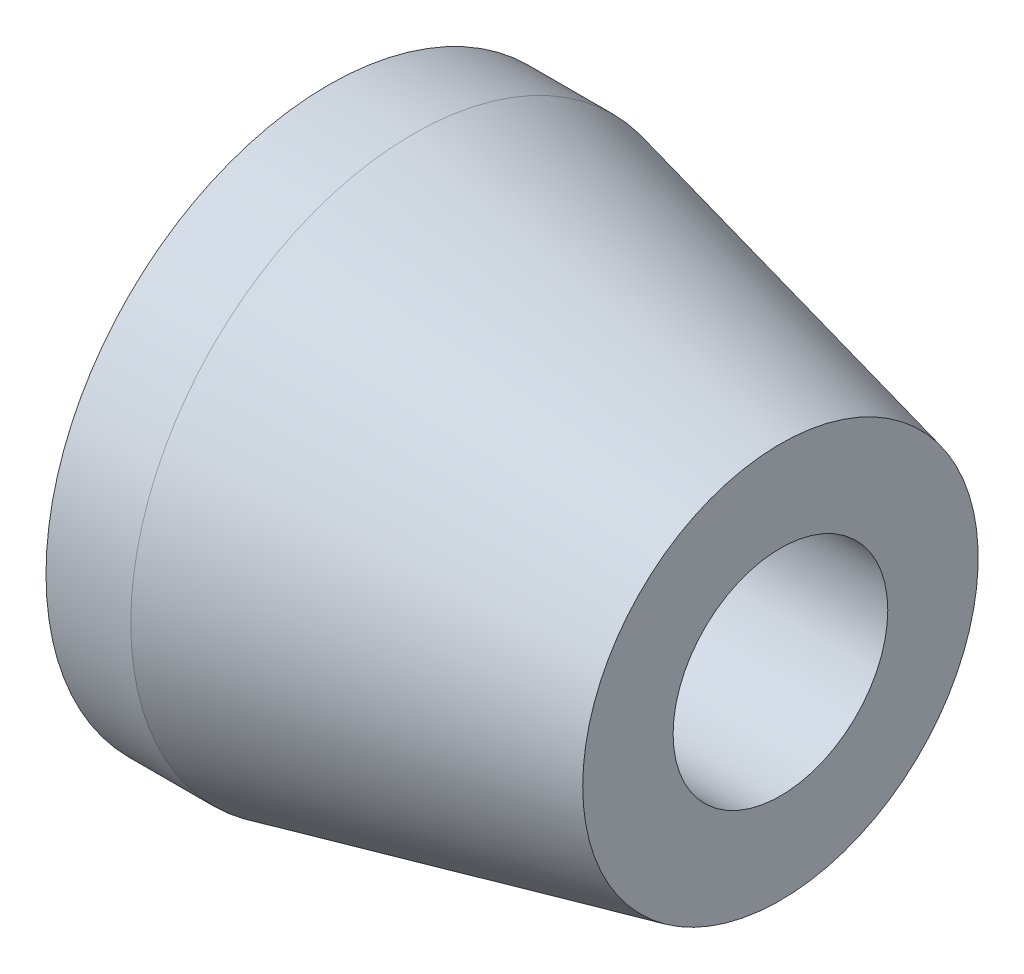
from build123d import *

# Parameters (mm, degrees)
BORE_SKETCH_R      = 3.8
THROUGH_BORE_DEPTH = 22.354156504
RECESS_SKETCH_13_R = 6.5
RECESS_13X2_DEPTH  = 2


with BuildPart() as part:
    # Bush Profile Sketch → Bush Body (revolve)
    with BuildSketch(Plane.XY, mode=Mode.PRIVATE) as bush_body_sk:
        Polygon((0, 0), (0, 10), (3, 10), (16, 7), (16, 0), align=None)
    revolve(bush_body_sk.sketch.rotate(Axis((-1000, 0, 0), (1, 0, 0)), 90), axis=Axis((-1000, 0, 0), (1, 0, 0)))

    # Bore Sketch → Through Bore (cut, through all)
    with BuildSketch(Plane.ZY):
        Circle(BORE_SKETCH_R)
    extrude(amount=-THROUGH_BORE_DEPTH, mode=Mode.SUBTRACT)

    # Recess Sketch Ø13 → Recess Ø13x2 (cut)
    with BuildSketch(Plane.ZY):
        Circle(RECESS_SKETCH_13_R)
    extrude(amount=-RECESS_13X2_DEPTH, mode=Mode.SUBTRACT)


solid = part.part
